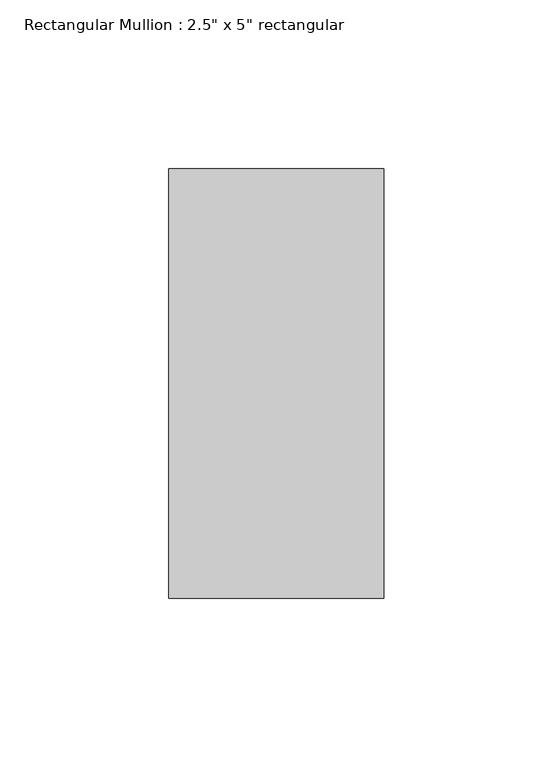
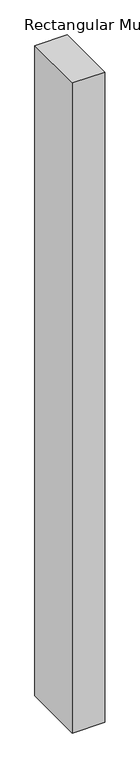
"""IFC4 building model written with IfcOpenShell, lengths in millimetres: member geometry."""

from ifc_helpers import new_model, si_unit, frame, origin, place, context, project, spatial, polyline, outline, extrude, source, transform, mapped, element, save


def member_01694e6c(model_context):
    return source(origin(), model_context, "Body", "SweptSolid", [
        extrude(outline(polyline([(0.0, 63.5), (0.0, -63.5), (-63.5, -63.5), (-63.5, 63.5), (0.0, 63.5)])), frame((0.0, 0.0, -1349.975361), z_axis=(0.0, 0.0, 1.0), x_axis=(1.0, 0.0, 0.0)), (0.0, 0.0, 1.0), 1349.975361),
    ])


if __name__ == "__main__":
    model = new_model("IFC4")
    model_context = context("Model", 3, world=origin())
    ifc_project = project(units=[si_unit("LENGTHUNIT", "METRE", prefix="MILLI")], contexts=[model_context])
    site = spatial("IfcSite", under=ifc_project)
    building = spatial("IfcBuilding", under=site)
    placement = place(None, origin())
    member_shape = member_01694e6c(model_context)
    element("IfcMember", 1, ObjectType="Rectangular Mullion : 2.5\" x 5\" rectangular", at=placement, inside=building, context=model_context, shape_type="MappedRepresentation", body=[
        mapped(member_shape, transform((0.0, 0.0, 0.0), x_axis=(1.0, 0.0, 0.0), y_axis=(0.0, 1.0, 0.0), z_axis=(0.0, 0.0, 1.0))),
    ])
    save(model, "model.ifc")

# Revit data of these elements
# Type "Rectangular Mullion : 2.5\" x 5\" rectangular"
#   built-in parameter 1007304 = 0.416667 (stored number, unit not read)
#   built-in parameter 1007301 = 0.104167 (stored number, unit not read)
#   built-in parameter 1007300 = 0.104167 (stored number, unit not read)
# Element 1 (IfcMember, "Rectangular Mullion : 2.5\" x 5\" rectangular")
#   Materials on its faces: "Aluminum"
# Materials
#   "Aluminum": class "Metal", colour RGB 247 247 247, transparency 0, Description = "Aluminum 6061", Cost = 0
